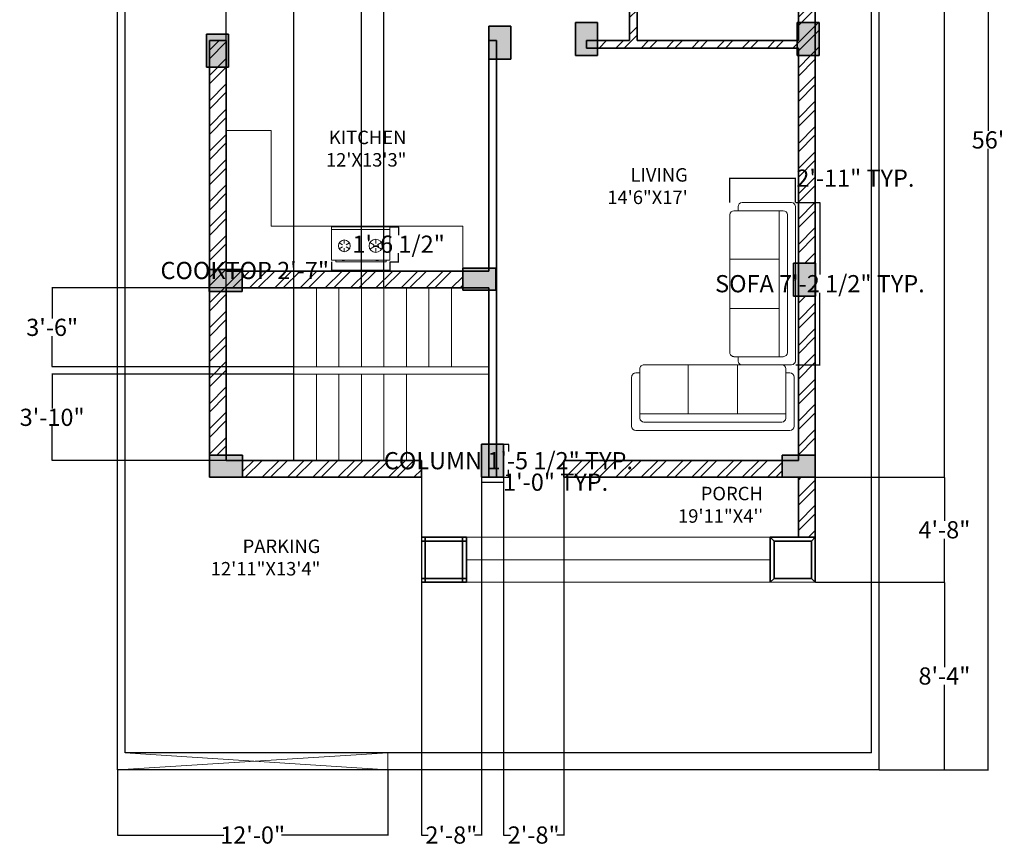
# Model space of a CAD drawing. Units: inches. Extents: x 104 to 629, y 1868 to 5138.
# Tile 1 of 2: x 104 to 629, y 1868 to 2309. Entities that reach past the tile are written whole.
import ezdxf

# ---------------------------------------------------------------- set-up
doc = ezdxf.new("R2010")
doc.units = ezdxf.units.IN
for name, color, linetype, lineweight in [('00 FURNITURE', 15, 'Continuous', 15), ('A-ANNO-DIMS', 2, 'Continuous', 18), ('A-AREA-IDEN', 7, 'Continuous', 18), ('A-EQPM', 8, 'Continuous', 18), ('A-FLOR-CASE', 8, 'Continuous', 18), ('A-FLOR-STRS', 7, 'Continuous', 18), ('A-WALL-PATT', 8, 'Continuous', 13), ('C-PROP', 7, 'Continuous', 25), ('C-SITE-GATE', 4, 'Continuous', 18), ('column', 10, 'Continuous', 35), ('hatch column', 10, 'Continuous', 13), ('WALL', 7, 'Continuous', 35)]:
    doc.layers.add(name, color=color, linetype=linetype, lineweight=lineweight)
doc.layers.add('FURN3D', color=229, linetype='Continuous', lineweight=5, true_color=0x4a3f41)
doc.styles.get("Standard").update_dxf_attribs({"font": 'arial.ttf'})
doc.dimstyles.get("Standard").update_dxf_attribs({"dimtxt": 9.18, "dimasz": 0.18, "dimexe": 0.18, "dimexo": 0.0625, "dimgap": 0.09, "dimtad": 0, "dimtih": 1, "dimtoh": 1, "dimdec": 1, "dimzin": 0, "dimdsep": 46, "dimlunit": 3, "dimtxsty": 'Standard', "dimcen": 0.09, "dimadec": 0, "dimazin": 0, "dimtfac": 1, "dimtdec": 1, "dimtofl": 0, "dimtmove": 0, "dimatfit": 3, "dimfxl": 1, "dimtolj": 1, "dimtzin": 0, "dimarcsym": 0})

# ---------------------------------------------------------------- blocks, each defined once
blk = doc.blocks.new('column')
at = {"layer": 'column'}
for p, q in [((661.29, 2690.99), (673.05, 2690.99)), ((661.29, 2673.35), (661.29, 2690.99)), ((673.05, 2690.99), (673.05, 2673.35)), ((673.05, 2673.35), (661.29, 2673.35))]:
    blk.add_line(p, q, dxfattribs=at)
blk = doc.blocks.new('A$C21540130')
at = {"layer": 'FURN3D'}
for p, q in [((1.57, 0), (1.57, 31.11)), ((9.61, 25.31), (8.63, 27.01)), ((10.79, 25.31), (11.77, 27.01)), ((9.02, 24.29, -27.54), (7.06, 24.29, -27.54)), ((9.61, 23.27), (8.63, 21.57)), ((10.79, 23.27), (11.77, 21.57)), ((11.38, 24.29, -27.54), (13.34, 24.29, -27.54)), ((9.61, 8.56), (8.43, 10.6)), ((10.79, 8.56), (11.97, 10.6)), ((9.02, 7.54), (6.67, 7.54)), ((9.61, 6.52), (8.43, 4.48)), ((10.79, 6.52), (11.97, 4.48)), ((11.38, 7.54), (13.73, 7.54))]:
    blk.add_line(p, q, dxfattribs=at)
for points in [[(0, 0), (0, 31.11), (17.9, 31.11), (17.9, 0)], [(18.68, 1.96), (18.68, 28.83), (17.9, 28.83), (17.9, 1.96)]]:
    blk.add_lwpolyline(points, close=True, dxfattribs=at)
for centre, radius in [((10.2, 24.29), 3.14), ((10.2, 7.54), 3.53)]:
    blk.add_circle(centre, radius, dxfattribs=at)
for points in [[(17.9, 24.03), (18.29, 24.03), (17.9, 25.6), (18.29, 25.6)], [(17.9, 6.05), (18.29, 6.05), (17.9, 7.62), (18.29, 7.62)]]:
    blk.add_solid(points, dxfattribs=at)
blk = doc.blocks.new('sofa 6')
for p, q in [((-1100, 167), (-1100, 834)), ((-1044, 890), (1044, 890)), ((1100, 834), (1100, 167)), ((-989, 56), (-989, 723)), ((-989, 667), (989, 667)), ((-933, 779), (933, 779)), ((-334, 667), (-334, 0)), ((334, 667), (334, 0)), ((989, 723), (989, 56)), ((-989, 111), (-1044, 111)), ((933, 0), (-933, 0)), ((1044, 111), (989, 111))]:
    blk.add_line(p, q)
for centre, start, end in [((-1044, 834), 90, 180), ((1044, 834), 0, 90), ((-933, 723), 90, 180), ((933, 723), 0, 90), ((-1044, 167), 180, 270), ((1044, 167), 270, 0), ((-933, 56), 180, 270), ((933, 56), 270, 0)]:
    blk.add_arc(centre, 55.6, start, end)
blk = doc.blocks.new('*D14')
at = {"layer": 'A-ANNO-DIMS', "color": 0, "lineweight": -2, "transparency": 16777216}
for p, q in [((561.97, 2580.99), (620.18, 2580.99)), ((620, 2580.81), (620, 2249.77)), ((620, 1909.17), (620, 2240.21)), ((561.97, 1908.99), (620.18, 1908.99))]:
    blk.add_line(p, q, dxfattribs=at)
at = {"layer": 'A-ANNO-DIMS', "color": 0, "transparency": 16777216}
for points in [[(619.97, 2580.81), (620.03, 2580.81), (620, 2580.99)], [(619.97, 1909.17), (620.03, 1909.17), (620, 1908.99)]]:
    blk.add_solid(points, dxfattribs=at)
at = {"layer": 'Defpoints', "color": 0, "transparency": 16777216}
for p in [(561.91, 2580.99), (561.91, 1908.99), (620, 1908.99)]:
    blk.add_point(p, dxfattribs=at)
at = {"layer": 'A-ANNO-DIMS', "color": 0, "transparency": 16777216, "insert": (620, 2244.99), "char_height": 9.18, "attachment_point": 5}
blk.add_mtext("\\A1;56'", dxfattribs=at)
blk = doc.blocks.new('*D15')
at = {"layer": 'A-ANNO-DIMS', "color": 0, "lineweight": -2, "transparency": 16777216}
for p, q in [((361.74, 2082.67), (364.5, 2082.67)), ((364.32, 2082.49), (364.32, 2078.69)), ((364.32, 2065.21), (364.32, 2069.01)), ((361.74, 2065.03), (364.5, 2065.03))]:
    blk.add_line(p, q, dxfattribs=at)
at = {"layer": 'A-ANNO-DIMS', "color": 0, "transparency": 16777216}
for points in [[(364.29, 2082.49), (364.35, 2082.49), (364.32, 2082.67)], [(364.29, 2065.21), (364.35, 2065.21), (364.32, 2065.03)]]:
    blk.add_solid(points, dxfattribs=at)
at = {"layer": 'Defpoints', "color": 0, "transparency": 16777216}
for p in [(361.68, 2082.67), (364.32, 2082.67), (361.68, 2065.03)]:
    blk.add_point(p, dxfattribs=at)
at = {"layer": 'A-ANNO-DIMS', "color": 0, "transparency": 16777216, "insert": (364.32, 2073.85), "char_height": 9.18, "attachment_point": 5}
blk.add_mtext('\\A1;COLUMN 1\'-5 1/2" TYP.', dxfattribs=at)
blk = doc.blocks.new('*D16')
at = {"layer": 'A-ANNO-DIMS', "color": 0, "lineweight": -2, "transparency": 16777216}
for p, q in [((349.92, 2064.97), (349.92, 2062.21)), ((361.68, 2064.97), (361.68, 2062.21)), ((350.1, 2062.39), (361.5, 2062.39)), ((361.68, 2062.39), (361.86, 2062.39))]:
    blk.add_line(p, q, dxfattribs=at)
at = {"layer": 'A-ANNO-DIMS', "color": 0, "transparency": 16777216}
for points in [[(350.1, 2062.42), (350.1, 2062.36), (349.92, 2062.39)], [(361.5, 2062.42), (361.5, 2062.36), (361.68, 2062.39)]]:
    blk.add_solid(points, dxfattribs=at)
at = {"layer": 'Defpoints', "color": 0, "transparency": 16777216}
for p in [(349.92, 2065.03), (361.68, 2065.03), (361.68, 2062.39)]:
    blk.add_point(p, dxfattribs=at)
at = {"layer": 'A-ANNO-DIMS', "color": 0, "transparency": 16777216, "insert": (389.49, 2062.39), "char_height": 9.18, "attachment_point": 5}
blk.add_mtext('\\A1;1\'-0" TYP.', dxfattribs=at)
blk = doc.blocks.new('*D19')
at = {"layer": 'A-ANNO-DIMS', "color": 0, "lineweight": -2, "transparency": 16777216}
for p, q in [((517.46, 2211.59), (530.57, 2211.59)), ((530.39, 2211.41), (530.39, 2173.12)), ((530.39, 2125.15), (530.39, 2163.44)), ((517.46, 2124.97), (530.57, 2124.97))]:
    blk.add_line(p, q, dxfattribs=at)
at = {"layer": 'A-ANNO-DIMS', "color": 0, "transparency": 16777216}
for points in [[(530.36, 2211.41), (530.42, 2211.41), (530.39, 2211.59)], [(530.36, 2125.15), (530.42, 2125.15), (530.39, 2124.97)]]:
    blk.add_solid(points, dxfattribs=at)
at = {"layer": 'Defpoints', "color": 0, "transparency": 16777216}
for p in [(517.4, 2211.59), (517.4, 2124.97), (530.39, 2124.97)]:
    blk.add_point(p, dxfattribs=at)
at = {"layer": 'A-ANNO-DIMS', "color": 0, "transparency": 16777216, "insert": (530.39, 2168.28), "char_height": 9.18, "attachment_point": 5}
blk.add_mtext('\\A1;SOFA 7\'-2 1/2" TYP.', dxfattribs=at)
blk = doc.blocks.new('*D20')
at = {"layer": 'A-ANNO-DIMS', "color": 0, "lineweight": -2, "transparency": 16777216}
for p, q in [((482.36, 2211.65), (482.36, 2224.76)), ((482.54, 2224.58), (517.22, 2224.58)), ((517.4, 2211.65), (517.4, 2224.76)), ((517.4, 2224.58), (517.58, 2224.58))]:
    blk.add_line(p, q, dxfattribs=at)
at = {"layer": 'A-ANNO-DIMS', "color": 0, "transparency": 16777216}
for points in [[(482.54, 2224.61), (482.54, 2224.55), (482.36, 2224.58)], [(517.22, 2224.61), (517.22, 2224.55), (517.4, 2224.58)]]:
    blk.add_solid(points, dxfattribs=at)
at = {"layer": 'Defpoints', "color": 0, "transparency": 16777216}
for p in [(517.4, 2224.58), (482.36, 2211.59), (517.4, 2211.59)]:
    blk.add_point(p, dxfattribs=at)
at = {"layer": 'A-ANNO-DIMS', "color": 0, "transparency": 16777216, "insert": (549.29, 2224.58), "char_height": 9.18, "attachment_point": 5}
blk.add_mtext('\\A1;2\'-11" TYP.', dxfattribs=at)
blk = doc.blocks.new('*D21')
at = {"layer": 'A-ANNO-DIMS', "color": 0, "lineweight": -2, "transparency": 16777216}
for p, q in [((270, 2179.94), (270, 2175.15)), ((301.11, 2179.94), (301.11, 2175.15)), ((270, 2175.33), (269.82, 2175.33)), ((300.93, 2175.33), (270.18, 2175.33))]:
    blk.add_line(p, q, dxfattribs=at)
at = {"layer": 'A-ANNO-DIMS', "color": 0, "transparency": 16777216}
for points in [[(270.18, 2175.36), (270.18, 2175.3), (270, 2175.33)], [(300.93, 2175.36), (300.93, 2175.3), (301.11, 2175.33)]]:
    blk.add_solid(points, dxfattribs=at)
at = {"layer": 'Defpoints', "color": 0, "transparency": 16777216}
for p in [(270, 2180), (301.11, 2180), (270, 2175.33)]:
    blk.add_point(p, dxfattribs=at)
at = {"layer": 'A-ANNO-DIMS', "color": 0, "transparency": 16777216, "insert": (223.74, 2175.33), "char_height": 9.18, "attachment_point": 5}
blk.add_mtext('\\A1;COOKTOP 2\'-7"', dxfattribs=at)
blk = doc.blocks.new('*D22')
at = {"layer": 'A-ANNO-DIMS', "color": 0, "lineweight": -2, "transparency": 16777216}
for p, q in [((301.17, 2198.68), (305.95, 2198.68)), ((305.77, 2198.5), (305.77, 2194.18)), ((305.77, 2180.18), (305.77, 2184.51)), ((301.17, 2180), (305.95, 2180))]:
    blk.add_line(p, q, dxfattribs=at)
at = {"layer": 'A-ANNO-DIMS', "color": 0, "transparency": 16777216}
for points in [[(305.74, 2198.5), (305.8, 2198.5), (305.77, 2198.68)], [(305.74, 2180.18), (305.8, 2180.18), (305.77, 2180)]]:
    blk.add_solid(points, dxfattribs=at)
at = {"layer": 'Defpoints', "color": 0, "transparency": 16777216}
for p in [(301.11, 2198.68), (301.11, 2180), (305.77, 2180)]:
    blk.add_point(p, dxfattribs=at)
at = {"layer": 'A-ANNO-DIMS', "color": 0, "transparency": 16777216, "insert": (305.77, 2189.34), "char_height": 9.18, "attachment_point": 5}
blk.add_mtext('\\A1;1\'-6 1/2"', dxfattribs=at)
blk = doc.blocks.new('*D27')
at = {"layer": 'A-ANNO-DIMS', "color": 0, "lineweight": -2, "transparency": 16777216}
for p, q in [((405.93, 2580.97), (596.94, 2580.97)), ((596.76, 2580.79), (596.76, 2327.76)), ((596.76, 2065.18), (596.76, 2318.2)), ((527.99, 2065), (596.94, 2065))]:
    blk.add_line(p, q, dxfattribs=at)
at = {"layer": 'A-ANNO-DIMS', "color": 0, "transparency": 16777216}
for points in [[(596.73, 2580.79), (596.79, 2580.79), (596.76, 2580.97)], [(596.73, 2065.18), (596.79, 2065.18), (596.76, 2065)]]:
    blk.add_solid(points, dxfattribs=at)
at = {"layer": 'Defpoints', "color": 0, "transparency": 16777216}
for p in [(405.87, 2580.97), (596.76, 2580.97), (527.93, 2065)]:
    blk.add_point(p, dxfattribs=at)
at = {"layer": 'A-ANNO-DIMS', "color": 0, "transparency": 16777216, "insert": (596.76, 2322.98), "char_height": 9.18, "attachment_point": 5}
blk.add_mtext('\\A1;43\'-0"', dxfattribs=at)
blk = doc.blocks.new('*D28')
at = {"layer": 'A-ANNO-DIMS', "color": 0, "lineweight": -2, "transparency": 16777216}
for p, q in [((527.99, 2065), (596.94, 2065)), ((596.76, 2064.82), (596.76, 2041.77)), ((596.76, 2009.17), (596.76, 2032.22)), ((527.97, 2008.99), (596.94, 2008.99))]:
    blk.add_line(p, q, dxfattribs=at)
at = {"layer": 'A-ANNO-DIMS', "color": 0, "transparency": 16777216}
for points in [[(596.73, 2064.82), (596.79, 2064.82), (596.76, 2065)], [(596.73, 2009.17), (596.79, 2009.17), (596.76, 2008.99)]]:
    blk.add_solid(points, dxfattribs=at)
at = {"layer": 'Defpoints', "color": 0, "transparency": 16777216}
for p in [(527.93, 2065), (596.76, 2065), (527.91, 2008.99)]:
    blk.add_point(p, dxfattribs=at)
at = {"layer": 'A-ANNO-DIMS', "color": 0, "transparency": 16777216, "insert": (596.76, 2036.99), "char_height": 9.18, "attachment_point": 5}
blk.add_mtext('\\A1;4\'-8"', dxfattribs=at)
blk = doc.blocks.new('*D29')
at = {"layer": 'A-ANNO-DIMS', "color": 0, "lineweight": -2, "transparency": 16777216}
for p, q in [((527.97, 2008.99), (596.94, 2008.99)), ((596.76, 2008.81), (596.76, 1963.77)), ((596.76, 1909.17), (596.76, 1954.21)), ((561.97, 1908.99), (596.94, 1908.99))]:
    blk.add_line(p, q, dxfattribs=at)
at = {"layer": 'A-ANNO-DIMS', "color": 0, "transparency": 16777216}
for points in [[(596.73, 2008.81), (596.79, 2008.81), (596.76, 2008.99)], [(596.73, 1909.17), (596.79, 1909.17), (596.76, 1908.99)]]:
    blk.add_solid(points, dxfattribs=at)
at = {"layer": 'Defpoints', "color": 0, "transparency": 16777216}
for p in [(527.91, 2008.99), (596.76, 2008.99), (561.91, 1908.99)]:
    blk.add_point(p, dxfattribs=at)
at = {"layer": 'A-ANNO-DIMS', "color": 0, "transparency": 16777216, "insert": (596.76, 1958.99), "char_height": 9.18, "attachment_point": 5}
blk.add_mtext('\\A1;8\'-4"', dxfattribs=at)
blk = doc.blocks.new('*D30')
at = {"layer": 'A-ANNO-DIMS', "color": 0, "lineweight": -2, "transparency": 16777216}
for p, q in [((155.91, 1908.93), (155.91, 1873.96)), ((300, 1908.93), (300, 1873.96)), ((156.09, 1874.14), (212.53, 1874.14)), ((299.82, 1874.14), (243.38, 1874.14))]:
    blk.add_line(p, q, dxfattribs=at)
at = {"layer": 'A-ANNO-DIMS', "color": 0, "transparency": 16777216}
for points in [[(156.09, 1874.17), (156.09, 1874.11), (155.91, 1874.14)], [(299.82, 1874.17), (299.82, 1874.11), (300, 1874.14)]]:
    blk.add_solid(points, dxfattribs=at)
at = {"layer": 'Defpoints', "color": 0, "transparency": 16777216}
for p in [(155.91, 1908.99), (300, 1908.99), (300, 1874.14)]:
    blk.add_point(p, dxfattribs=at)
at = {"layer": 'A-ANNO-DIMS', "color": 0, "transparency": 16777216, "insert": (227.95, 1874.14), "char_height": 9.18, "attachment_point": 5}
blk.add_mtext('\\A1;12\'-0"', dxfattribs=at)
blk = doc.blocks.new('*D31')
at = {"layer": 'A-ANNO-DIMS', "color": 0, "lineweight": -2, "transparency": 16777216}
for p, q in [((213.91, 2074.05), (213.91, 2617.21)), ((214.09, 2617.03), (219.62, 2617.03)), ((249.73, 2617.03), (244.2, 2617.03)), ((249.91, 2074.05), (249.91, 2617.21))]:
    blk.add_line(p, q, dxfattribs=at)
at = {"layer": 'A-ANNO-DIMS', "color": 0, "transparency": 16777216}
for points in [[(214.09, 2617.06), (214.09, 2617), (213.91, 2617.03)], [(249.73, 2617.06), (249.73, 2617), (249.91, 2617.03)]]:
    blk.add_solid(points, dxfattribs=at)
at = {"layer": 'Defpoints', "color": 0, "transparency": 16777216}
for p in [(249.91, 2617.03), (213.91, 2073.99), (249.91, 2073.99)]:
    blk.add_point(p, dxfattribs=at)
at = {"layer": 'A-ANNO-DIMS', "color": 0, "transparency": 16777216, "insert": (231.91, 2617.03), "char_height": 9.18, "attachment_point": 5}
blk.add_mtext('\\A1;3\'-0"', dxfattribs=at)
blk = doc.blocks.new('*D32')
at = {"layer": 'A-ANNO-DIMS', "color": 0, "lineweight": -2, "transparency": 16777216}
for p, q in [((249.85, 2165.99), (120.88, 2165.99)), ((121.06, 2165.81), (121.06, 2149.77)), ((121.06, 2124.17), (121.06, 2140.21)), ((249.85, 2123.99), (120.88, 2123.99))]:
    blk.add_line(p, q, dxfattribs=at)
at = {"layer": 'A-ANNO-DIMS', "color": 0, "transparency": 16777216}
for points in [[(121.03, 2165.81), (121.09, 2165.81), (121.06, 2165.99)], [(121.03, 2124.17), (121.09, 2124.17), (121.06, 2123.99)]]:
    blk.add_solid(points, dxfattribs=at)
at = {"layer": 'Defpoints', "color": 0, "transparency": 16777216}
for p in [(121.06, 2165.99), (249.91, 2165.99), (249.91, 2123.99)]:
    blk.add_point(p, dxfattribs=at)
at = {"layer": 'A-ANNO-DIMS', "color": 0, "transparency": 16777216, "insert": (121.06, 2144.99), "char_height": 9.18, "attachment_point": 5}
blk.add_mtext('\\A1;3\'-6"', dxfattribs=at)
blk = doc.blocks.new('*D33')
at = {"layer": 'A-ANNO-DIMS', "color": 0, "lineweight": -2, "transparency": 16777216}
for p, q in [((249.85, 2119.99), (120.88, 2119.99)), ((121.06, 2119.81), (121.06, 2101.77)), ((121.06, 2074.17), (121.06, 2092.21)), ((249.85, 2073.99), (120.88, 2073.99))]:
    blk.add_line(p, q, dxfattribs=at)
at = {"layer": 'A-ANNO-DIMS', "color": 0, "transparency": 16777216}
for points in [[(121.03, 2119.81), (121.09, 2119.81), (121.06, 2119.99)], [(121.03, 2074.17), (121.09, 2074.17), (121.06, 2073.99)]]:
    blk.add_solid(points, dxfattribs=at)
at = {"layer": 'Defpoints', "color": 0, "transparency": 16777216}
for p in [(121.06, 2119.99), (249.91, 2119.99), (249.91, 2073.99)]:
    blk.add_point(p, dxfattribs=at)
at = {"layer": 'A-ANNO-DIMS', "color": 0, "transparency": 16777216, "insert": (121.06, 2096.99), "char_height": 9.18, "attachment_point": 5}
blk.add_mtext('\\A1;3\'-10"', dxfattribs=at)
blk = doc.blocks.new('*D34')
at = {"layer": 'A-ANNO-DIMS', "color": 0, "lineweight": -2, "transparency": 16777216}
for p, q in [((361.68, 2064.97), (361.68, 1873.96)), ((393.91, 2064.93), (393.91, 1873.96)), ((361.86, 1874.14), (365.42, 1874.14)), ((393.73, 1874.14), (390.16, 1874.14))]:
    blk.add_line(p, q, dxfattribs=at)
at = {"layer": 'A-ANNO-DIMS', "color": 0, "transparency": 16777216}
for points in [[(361.86, 1874.17), (361.86, 1874.11), (361.68, 1874.14)], [(393.73, 1874.17), (393.73, 1874.11), (393.91, 1874.14)]]:
    blk.add_solid(points, dxfattribs=at)
at = {"layer": 'Defpoints', "color": 0, "transparency": 16777216}
for p in [(361.68, 2065.03), (393.91, 2064.99), (393.91, 1874.14)]:
    blk.add_point(p, dxfattribs=at)
at = {"layer": 'A-ANNO-DIMS', "color": 0, "transparency": 16777216, "insert": (377.79, 1874.14), "char_height": 9.18, "attachment_point": 5}
blk.add_mtext('\\A1;2\'-8"', dxfattribs=at)
blk = doc.blocks.new('*D35')
at = {"layer": 'A-ANNO-DIMS', "color": 0, "lineweight": -2, "transparency": 16777216}
for p, q in [((317.91, 2064.93), (317.91, 1873.96)), ((349.92, 2064.97), (349.92, 1873.96)), ((318.09, 1874.14), (321.54, 1874.14)), ((349.74, 1874.14), (346.28, 1874.14))]:
    blk.add_line(p, q, dxfattribs=at)
at = {"layer": 'A-ANNO-DIMS', "color": 0, "transparency": 16777216}
for points in [[(318.09, 1874.17), (318.09, 1874.11), (317.91, 1874.14)], [(349.74, 1874.17), (349.74, 1874.11), (349.92, 1874.14)]]:
    blk.add_solid(points, dxfattribs=at)
at = {"layer": 'Defpoints', "color": 0, "transparency": 16777216}
for p in [(317.91, 2064.99), (349.92, 2065.03), (349.92, 1874.14)]:
    blk.add_point(p, dxfattribs=at)
at = {"layer": 'A-ANNO-DIMS', "color": 0, "transparency": 16777216, "insert": (333.91, 1874.14), "char_height": 9.18, "attachment_point": 5}
blk.add_mtext('\\A1;2\'-8"', dxfattribs=at)
blk = doc.blocks.new('*D36')
at = {"layer": 'A-ANNO-DIMS', "color": 0, "lineweight": -2, "transparency": 16777216}
for p, q in [((285.91, 2166.05), (285.91, 2617.21)), ((286.09, 2617.03), (297.73, 2617.03)), ((297.91, 2166.05), (297.91, 2617.21)), ((297.91, 2617.03), (298.09, 2617.03))]:
    blk.add_line(p, q, dxfattribs=at)
at = {"layer": 'A-ANNO-DIMS', "color": 0, "transparency": 16777216}
for points in [[(286.09, 2617.06), (286.09, 2617), (285.91, 2617.03)], [(297.73, 2617.06), (297.73, 2617), (297.91, 2617.03)]]:
    blk.add_solid(points, dxfattribs=at)
at = {"layer": 'Defpoints', "color": 0, "transparency": 16777216}
for p in [(297.91, 2617.03), (285.91, 2165.99), (297.91, 2165.99)]:
    blk.add_point(p, dxfattribs=at)
at = {"layer": 'A-ANNO-DIMS', "color": 0, "transparency": 16777216, "insert": (309.95, 2617.03), "char_height": 9.18, "attachment_point": 5}
blk.add_mtext('\\A1;1\'-0"', dxfattribs=at)

msp = doc.modelspace()

# ---------------------------------------------------------------- hatches: boundary and pattern name
at = {"layer": 'A-WALL-PATT'}
h = msp.add_hatch(dxfattribs=at)
h.set_pattern_fill('ANSI32', color=256)
h.paths.add_polyline_path([(527.91, 2307.64), (530, 2307.64), (530, 2290), (518.24, 2290), (518.24, 2307.64), (518.91, 2307.64), (518.91, 2345.99), (466.91, 2345.99), (466.91, 2363.99), (470.91, 2363.99), (470.91, 2349.99), (518.91, 2349.99), (518.91, 2393.99), (431.91, 2393.99), (431.91, 2397.99), (518.91, 2397.99), (518.91, 2436.87), (515.84, 2436.87), (515.84, 2454.51), (527.91, 2454.51)])
h.paths.add_polyline_path([(432.91, 2345.99), (436.91, 2345.99), (436.91, 2349.99), (428.91, 2349.99), (428.91, 2297.99), (411.76, 2297.99), (411.76, 2293.99), (518.24, 2293.99), (518.24, 2297.99), (432.91, 2297.99)])
h = msp.add_hatch(dxfattribs=at)
h.set_pattern_fill('ANSI32', color=256)
h.paths.add_polyline_path([(317.91, 2073.99), (222.56, 2073.99), (222.56, 2064.99), (317.91, 2064.99)])
h.paths.add_polyline_path([(340.03, 2174.99), (222.37, 2174.99), (222.37, 2165.99), (340.03, 2165.99)])
h.paths.add_polyline_path([(213.91, 2164.12), (204.91, 2164.12), (204.91, 2076.76), (213.91, 2076.76)])
h.paths.add_polyline_path([(213.91, 2297.99), (204.91, 2297.99), (204.91, 2164.12), (213.91, 2164.12), (213.91, 2165.99), (222.37, 2165.99), (222.37, 2174.99), (213.91, 2174.99)])
h = msp.add_hatch(dxfattribs=at)
h.set_pattern_fill('ANSI32', color=256)
h.paths.add_polyline_path([(527.91, 2290), (518.91, 2290), (518.91, 2179.27), (527.91, 2179.27)])
h.paths.add_polyline_path([(527.91, 2161.63), (518.91, 2161.63), (518.91, 2076.76), (527.91, 2076.76)])
h.paths.add_polyline_path([(527.91, 2065), (518.91, 2065), (518.91, 2032.99), (527.91, 2032.99)])
h = msp.add_hatch(dxfattribs=at)
h.set_pattern_fill('ANSI32', color=256)
h.paths.add_polyline_path([(510.29, 2073.99), (393.91, 2073.99), (393.91, 2064.99), (510.29, 2064.99)])
at = {"layer": 'hatch column', "transparency": 33554559}
h = msp.add_hatch(color=256, dxfattribs=at)
h.dxf.hatch_style = 1
h.paths.add_polyline_path([(353.91, 2287.99), (365.67, 2287.99), (365.67, 2305.63), (353.91, 2305.63)])
h = msp.add_hatch(color=256, dxfattribs=at)
h.dxf.hatch_style = 1
h.paths.add_polyline_path([(411.76, 2307.64), (400, 2307.64), (400, 2290), (411.76, 2290)])
h = msp.add_hatch(color=256, dxfattribs=at)
h.dxf.hatch_style = 1
h.paths.add_polyline_path([(518.24, 2290), (530, 2290), (530, 2307.64), (518.24, 2307.64)])
h = msp.add_hatch(color=256, dxfattribs=at)
h.dxf.hatch_style = 1
h.paths.add_polyline_path([(203.28, 2283.8), (215.04, 2283.8), (215.04, 2301.44), (203.28, 2301.44)])
h = msp.add_hatch(color=256, dxfattribs=at)
h.dxf.hatch_style = 1
h.paths.add_polyline_path([(516.33, 2161.63), (528.09, 2161.63), (528.09, 2179.27), (516.33, 2179.27)])
h = msp.add_hatch(color=256, dxfattribs=at)
h.dxf.hatch_style = 1
h.paths.add_polyline_path([(204.73, 2175.88), (204.73, 2164.12), (222.37, 2164.12), (222.37, 2175.88)])
h = msp.add_hatch(color=256, dxfattribs=at)
h.dxf.hatch_style = 1
h.paths.add_polyline_path([(340.03, 2176.58), (340.03, 2164.82), (357.67, 2164.82), (357.67, 2176.58)])
h = msp.add_hatch(color=256, dxfattribs=at)
h.dxf.hatch_style = 1
h.paths.add_polyline_path([(349.92, 2065.03), (361.68, 2065.03), (361.68, 2082.67), (349.92, 2082.67)])
h = msp.add_hatch(color=256, dxfattribs=at)
h.dxf.hatch_style = 1
h.paths.add_polyline_path([(204.92, 2076.76), (204.92, 2065), (222.56, 2065), (222.56, 2076.76)])
h = msp.add_hatch(color=256, dxfattribs=at)
h.dxf.hatch_style = 1
h.paths.add_polyline_path([(510.29, 2076.76), (510.29, 2065), (527.93, 2065), (527.93, 2076.76)])

# ---------------------------------------------------------------- linework, layer by layer
at = {"layer": 'A-FLOR-CASE'}
for p, q in [((237.91, 2250), (213.91, 2250)), ((237.91, 2198.99), (237.91, 2250)), ((237.91, 2198.99), (340.03, 2198.99)), ((340.03, 2164.82), (340.03, 2198.99))]:
    msp.add_line(p, q, dxfattribs=at)
at = {"layer": 'A-FLOR-STRS'}
for p, q in [((249.91, 2073.99), (249.91, 2165.99)), ((261.91, 2123.99), (261.91, 2165.99)), ((273.91, 2123.99), (273.91, 2165.99)), ((285.91, 2123.99), (285.91, 2165.99)), ((297.91, 2123.99), (297.91, 2165.99)), ((309.91, 2123.99), (309.91, 2165.99)), ((321.91, 2123.99), (321.91, 2165.99)), ((333.91, 2123.99), (333.91, 2165.99)), ((249.91, 2123.99), (353.91, 2123.99)), ((249.91, 2119.99), (353.91, 2119.99)), ((261.91, 2073.99), (261.91, 2119.99)), ((273.91, 2073.99), (273.91, 2119.99)), ((285.91, 2073.99), (285.91, 2119.99)), ((297.91, 2073.99), (297.91, 2119.99)), ((309.91, 2073.99), (309.91, 2119.99)), ((317.91, 2064.99), (317.91, 2008.99)), ((317.91, 2032.99), (377.91, 2032.99)), ((353.91, 2032.99), (527.91, 2032.99)), ((341.91, 2020.99), (503.91, 2020.99)), ((317.91, 2008.99), (527.91, 2008.99))]:
    msp.add_line(p, q, dxfattribs=at)
at = {"layer": 'C-PROP'}
for p, q in [((155.91, 1908.99), (155.91, 2580.99)), ((561.91, 1908.99), (561.91, 2580.99)), ((159.91, 1917.99), (159.91, 2571.99)), ((557.91, 1917.99), (557.91, 2571.99)), ((557.91, 1917.99), (159.91, 1917.99)), ((561.91, 1908.99), (155.91, 1908.99))]:
    msp.add_line(p, q, dxfattribs=at)
at = {"layer": 'C-SITE-GATE'}
for p, q in [((155.91, 1908.99), (300, 1917.99)), ((300, 1908.99), (159.91, 1917.99)), ((300, 1917.99), (300, 1908.99))]:
    msp.add_line(p, q, dxfattribs=at)
at = {"layer": 'column'}
for p, q in [((317.91, 2032.99), (341.91, 2032.99)), ((319.91, 2032.99), (319.91, 2008.99)), ((339.91, 2032.99), (339.91, 2008.99)), ((341.91, 2032.99), (341.91, 2008.99)), ((527.91, 2032.99), (503.91, 2032.99)), ((503.91, 2032.99), (503.91, 2008.99)), ((503.91, 2032.99), (505.91, 2030.99)), ((527.91, 2032.99), (525.91, 2030.99)), ((317.91, 2030.99), (341.91, 2030.99)), ((505.91, 2030.99), (505.91, 2010.99)), ((525.91, 2030.99), (505.91, 2030.99)), ((525.91, 2010.99), (525.91, 2030.99)), ((317.91, 2010.99), (341.91, 2010.99)), ((503.91, 2008.99), (505.91, 2010.99)), ((505.91, 2010.99), (525.91, 2010.99)), ((527.91, 2008.99), (525.91, 2010.99)), ((317.91, 2008.99), (341.91, 2008.99))]:
    msp.add_line(p, q, dxfattribs=at)
at = {"layer": 'WALL'}
for p, q in [((527.91, 2008.99), (527.91, 2571.99)), ((428.91, 2297.99), (428.91, 2349.99)), ((432.91, 2297.99), (432.91, 2345.99)), ((518.91, 2297.99), (518.91, 2345.99)), ((204.91, 2064.99), (204.91, 2297.99)), ((213.91, 2297.99), (204.91, 2297.99)), ((213.91, 2174.99), (213.91, 2297.99)), ((357.91, 2297.99), (353.91, 2297.99)), ((353.91, 2174.99), (353.91, 2297.99)), ((357.91, 2080.99), (357.91, 2297.99)), ((405.91, 2297.99), (428.91, 2297.99)), ((405.91, 2293.99), (405.91, 2297.99)), ((432.91, 2297.99), (518.91, 2297.99)), ((405.91, 2293.99), (518.91, 2293.99)), ((518.91, 2073.99), (518.91, 2293.99)), ((213.91, 2174.99), (353.91, 2174.99)), ((213.91, 2165.99), (353.91, 2165.99)), ((213.91, 2073.99), (213.91, 2165.99)), ((353.91, 2064.99), (353.91, 2165.99)), ((357.91, 2064.99), (357.91, 2080.99)), ((518.91, 2073.99), (518.91, 2080.99)), ((317.91, 2073.99), (213.91, 2073.99)), ((317.91, 2064.99), (317.91, 2073.99)), ((518.91, 2073.99), (393.91, 2073.99)), ((393.91, 2064.99), (393.91, 2073.99)), ((317.91, 2064.99), (204.91, 2064.99)), ((357.91, 2064.99), (353.91, 2064.99)), ((518.91, 2064.99), (393.91, 2064.99)), ((518.91, 2032.99), (518.91, 2064.99)), ((518.91, 2032.99), (518.91, 2064.99))]:
    msp.add_line(p, q, dxfattribs=at)

# ---------------------------------------------------------------- block references
at = {"layer": '00 FURNITURE', "xscale": 0.0393700787401575, "yscale": 0.0393700787401575, "zscale": 0.0393700787401575}
for p, rotation in [((482.36, 2168.28), 270.0000000000005), ((473.31, 2125.04), 180)]:
    msp.add_blockref('sofa 6', p, dxfattribs=dict(at, rotation=rotation))
at = {"layer": 'A-EQPM', "xscale": -1, "rotation": 90}
msp.add_blockref('A$C21540130', (301.11, 2198.68), dxfattribs=at)
at = {"layer": 'column'}
for p in [(-307.38, -385.36), (-261.29, -383.35), (-143.05, -383.35), (-458.01, -389.56), (-144.97, -511.72), (-311.38, -608.32)]:
    msp.add_blockref('column', p, dxfattribs=at)
at = {"layer": 'column', "rotation": 270}
for p in [(-2468.62, 2837.17), (-2333.32, 2837.87), (-2468.43, 2738.05), (-2163.07, 2738.05)]:
    msp.add_blockref('column', p, dxfattribs=at)

# ---------------------------------------------------------------- texts
at = {"layer": 'A-AREA-IDEN', "attachment_point": 3}
for s, insert, char_height in [('KITCHEN\\P12\'X13\'3"', (309.94, 2249.92), 7.188), ('LIVING\\P14\'6"X17\'', (459.94, 2229.92), 7.188), ('PORCH\\P19\'11"X4\'{\\H0.83478x;\'}', (499.94, 2059.92), 7.1875), ('PARKING\\P12\'11"X13\'4"', (264.06, 2031.78), 7.1875)]:
    msp.add_mtext_dynamic_manual_height_columns(s, width=41.3807, gutter_width=12.5, heights=[0], dxfattribs=dict(at, insert=insert, char_height=char_height))

# ---------------------------------------------------------------- dimensions: what is measured, and where the dimension line sits
at = {"layer": 'A-ANNO-DIMS'}
for base, p1, p2, picture, middle in [((249.91, 2617.03), (213.91, 2073.99), (249.91, 2073.99), '*D31', (231.91, 2617.03)), ((297.91, 2617.03), (285.91, 2165.99), (297.91, 2165.99), '*D36', (309.95, 2617.03)), ((349.92, 1874.14), (317.91, 2064.99), (349.92, 2065.03), '*D35', (333.91, 1874.14)), ((393.91, 1874.14), (361.68, 2065.03), (393.91, 2064.99), '*D34', (377.79, 1874.14)), ((300, 1874.14), (155.91, 1908.99), (300, 1908.99), '*D30', (227.95, 1874.14))]:
    dim = msp.add_linear_dim(base=base, p1=p1, p2=p2, dimstyle='Standard', override={"dimdec": 1, "dimlfac": 1, "dimrnd": 0, "dimzin": 1, "dimdsep": 46, "dimlunit": 4, "dimfrac": 2}, dxfattribs=at)
    dim.commit()
    dim.dimension.update_dxf_attribs({"geometry": picture, "text_midpoint": middle})
for base, p1, p2, angle, override, picture, middle in [((596.76, 2580.97), (527.93, 2065), (405.87, 2580.97), 90, {"dimdec": 1, "dimlfac": 1, "dimrnd": 0, "dimzin": 1, "dimdsep": 46, "dimlunit": 4, "dimfrac": 2}, '*D27', (596.76, 2322.98)), ((620, 1908.99), (561.91, 2580.99), (561.91, 1908.99), 90, {"dimclrd": 0, "dimclre": 0, "dimclrt": 0}, '*D14', (620, 2244.99)), ((305.77, 2180), (301.11, 2198.68), (301.11, 2180), 270, {"dimdec": 1, "dimlfac": 1, "dimrnd": 0, "dimzin": 1, "dimdsep": 46, "dimlunit": 4, "dimfrac": 2}, '*D22', (305.77, 2189.34)), ((121.06, 2165.99), (249.91, 2123.99), (249.91, 2165.99), 90, {"dimdec": 1, "dimlfac": 1, "dimrnd": 0, "dimzin": 1, "dimdsep": 46, "dimlunit": 4, "dimfrac": 2}, '*D32', (121.06, 2144.99)), ((121.06, 2119.99), (249.91, 2073.99), (249.91, 2119.99), 90, {"dimdec": 1, "dimlfac": 1, "dimrnd": 0, "dimzin": 1, "dimdsep": 46, "dimlunit": 4, "dimfrac": 2}, '*D33', (121.06, 2096.99)), ((596.76, 2065), (527.91, 2008.99), (527.93, 2065), 90, {"dimdec": 1, "dimlfac": 1, "dimrnd": 0, "dimzin": 1, "dimdsep": 46, "dimlunit": 4, "dimfrac": 2}, '*D28', (596.76, 2036.99)), ((596.76, 2008.99), (561.91, 1908.99), (527.91, 2008.99), 90, {"dimdec": 1, "dimlfac": 1, "dimrnd": 0, "dimzin": 1, "dimdsep": 46, "dimlunit": 4, "dimfrac": 2}, '*D29', (596.76, 1958.99))]:
    dim = msp.add_linear_dim(base=base, p1=p1, p2=p2, angle=angle, dimstyle='Standard', override=override, dxfattribs=at)
    dim.commit()
    dim.dimension.update_dxf_attribs({"geometry": picture, "text_midpoint": middle})
for base, p1, p2, picture, middle in [((517.4, 2224.58), (482.36, 2211.59), (517.4, 2211.59), '*D20', (549.29, 2224.58)), ((361.68, 2062.39), (349.92, 2065.03), (361.68, 2065.03), '*D16', (389.49, 2062.39))]:
    dim = msp.add_linear_dim(base=base, p1=p1, p2=p2, text='<> TYP.', dimstyle='Standard', override={"dimdec": 1, "dimlfac": 1, "dimrnd": 0, "dimzin": 1, "dimdsep": 46, "dimlunit": 4, "dimfrac": 2}, dxfattribs=at)
    dim.commit()
    dim.dimension.update_dxf_attribs({"geometry": picture, "text_midpoint": middle})
for base, p1, p2, angle, text, picture, middle in [((530.39, 2124.97), (517.4, 2211.59), (517.4, 2124.97), 270, 'SOFA <> TYP.', '*D19', (530.39, 2168.28)), ((270, 2175.33), (301.11, 2180), (270, 2180), 180, 'COOKTOP <>', '*D21', (223.74, 2175.33)), ((364.32, 2082.67), (361.68, 2065.03), (361.68, 2082.67), 90, 'COLUMN <> TYP.', '*D15', (364.32, 2073.85))]:
    dim = msp.add_linear_dim(base=base, p1=p1, p2=p2, angle=angle, text=text, dimstyle='Standard', override={"dimdec": 1, "dimlfac": 1, "dimrnd": 0, "dimzin": 1, "dimdsep": 46, "dimlunit": 4, "dimfrac": 2}, dxfattribs=at)
    dim.commit()
    dim.dimension.update_dxf_attribs({"geometry": picture, "text_midpoint": middle})

doc.saveas('drawing.dxf')
